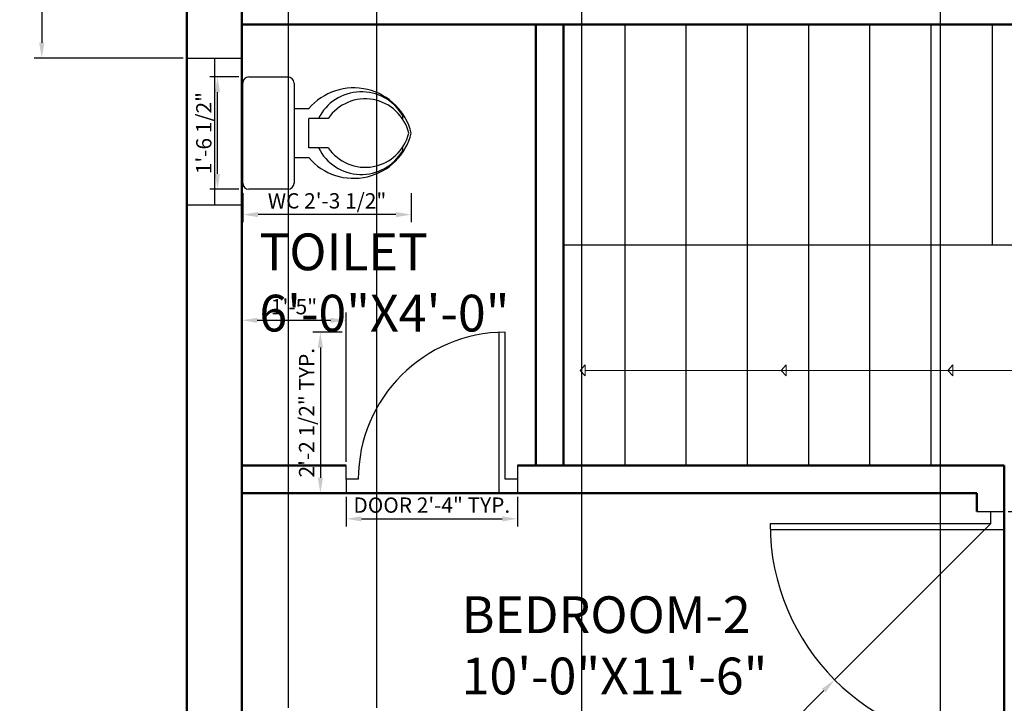
# Model space of a CAD drawing. Units: inches. Extents: x 3242 to 3618, y 1365 to 1814.
# Tile 2 of 6: x 3244 to 3405, y 1514 to 1626. Entities that reach past the tile are written whole.
import ezdxf

# ---------------------------------------------------------------- set-up
doc = ezdxf.new("R2010")
doc.units = ezdxf.units.IN
for name, color, linetype, lineweight in [('A-ANNO-DIMS', 2, 'Continuous', 18), ('A-ANNO-SYMB', 7, 'Continuous', 18), ('A-AREA-IDEN', 7, 'Continuous', 25), ('A-DOOR', 4, 'Continuous', 25), ('A-FLOR-FIXT', 8, 'Continuous', 25), ('A-FLOR-STRS', 7, 'Continuous', 25), ('A-GLAZ', 5, 'Continuous', 25), ('A-WALL', 7, 'Continuous', 50)]:
    doc.layers.add(name, color=color, linetype=linetype, lineweight=lineweight)
doc.styles.get("Standard").update_dxf_attribs({"font": 'arial.ttf'})
doc.dimstyles.new('ISO-25', dxfattribs={"dimtxt": 2.5, "dimasz": 2.5, "dimexe": 1.25, "dimexo": 0.625, "dimtad": 1, "dimdec": 0, "dimlunit": 3, "dimtxsty": 'Standard', "dimcen": 2.5, "dimadec": 0, "dimazin": 0, "dimtfac": 1, "dimtdec": 0, "dimtmove": 0, "dimatfit": 3, "dimfxl": 1, "dimarcsym": 0})

# ---------------------------------------------------------------- blocks, each defined once
blk = doc.blocks.new('A$C02F3725D')
for p, q in [((0.025, 0.69), (0.435, 0.69)), ((0, 0.505), (0, 0.665)), ((0.46, 0.665), (0.46, 0.505)), ((0.435, 0.48), (0.025, 0.48)), ((0.13, 0.48), (0.13, 0.42)), ((0.33, 0.42), (0.33, 0.48)), ((0.17, 0.34), (0.17, 0.42)), ((0.17, 0.42), (0.29, 0.42)), ((0.29, 0.34), (0.29, 0.42)), ((0.1578, 0.035), (0.1724, 0.035)), ((0.2876, 0.035), (0.3022, 0.035))]:
    blk.add_line(p, q)
for centre, radius, start, end in [((0.025, 0.665), 0.025, 90, 180), ((0.435, 0.665), 0.025, 0, 90), ((0.025, 0.505), 0.025, 180, 270), ((0.435, 0.505), 0.025, 270, 0), ((0.2874, 0.2356), 0.2425, 130.4885, 256.2965), ((0.1726, 0.2356), 0.2425, 283.7035, 49.5115), ((0.2568, 0.2042), 0.196, 116.2742, 239.6668), ((0.2032, 0.2042), 0.196, 300.3332, 63.7258), ((0.2732, 0.1883), 0.1834, 124.2157, 256.394), ((0.1868, 0.1883), 0.1834, 283.606, 55.7843)]:
    blk.add_arc(centre, radius, start, end)
blk = doc.blocks.new('DOOR-SWING-24IN')
for p, q in [((21.75, 28), (26.25, 28)), ((24, 28), (24, 26)), ((24, 26), (0, 26)), ((26.25, 25), (0, 25)), ((24, 2), (24, 0)), ((24, 0), (21.75, 0)), ((24, 0), (26.25, 0))]:
    blk.add_line(p, q)
blk.add_arc((24, 26), 24, 180, 270)
blk = doc.blocks.new('DOOR-SWING-36IN')
for p, q in [((33.75, 40), (38.25, 40)), ((36, 40), (36, 38)), ((36, 38), (0, 38)), ((38.25, 37), (0, 37)), ((36, 2), (36, 0)), ((36, 0), (33.75, 0)), ((36, 0), (38.25, 0))]:
    blk.add_line(p, q)
blk.add_arc((36, 38), 36, 180, 270)
blk = doc.blocks.new('WINDOW-24IN')
for p, q in [((0, 9), (24, 9)), ((0, 0), (0, 9)), ((24, 9), (24, 0)), ((0, 4.5), (24, 4.5)), ((24, 0), (0, 0))]:
    blk.add_line(p, q)
blk = doc.blocks.new('STAIR-DIR-ARROWHEAD')
for p, q in [((0.84, 1.76), (0, 0.88)), ((0.84, 0.88), (0.84, 1.76)), ((0.84, 0), (0, 0.88)), ((0.84, 0.88), (0.84, 0))]:
    blk.add_line(p, q)
blk = doc.blocks.new('*D17')
at = {"layer": 'A-ANNO-DIMS', "color": 0, "lineweight": -2, "transparency": 16777216}
for p, q in [((3405.61, 1545.66), (3412.23, 1545.66)), ((3410.98, 1508.16), (3410.98, 1543.16)), ((3405.61, 1505.66), (3412.23, 1505.66))]:
    blk.add_line(p, q, dxfattribs=at)
at = {"layer": 'A-ANNO-DIMS', "color": 0, "transparency": 16777216}
for points in [[(3410.56, 1543.16), (3411.4, 1543.16), (3410.98, 1545.66)], [(3410.56, 1508.16), (3411.4, 1508.16), (3410.98, 1505.66)]]:
    blk.add_solid(points, dxfattribs=at)
at = {"layer": 'Defpoints', "color": 0, "transparency": 16777216}
for p in [(3404.98, 1545.66), (3410.98, 1545.66), (3404.98, 1505.66)]:
    blk.add_point(p, dxfattribs=at)
at = {"layer": 'A-ANNO-DIMS', "color": 0, "transparency": 16777216, "insert": (3409.06, 1525.66), "char_height": 2.5, "attachment_point": 5, "rotation": 90}
blk.add_mtext('DOOR 3\'-4" TYP.', dxfattribs=at)
blk = doc.blocks.new('*D19')
at = {"layer": 'A-ANNO-DIMS', "color": 0, "lineweight": -2, "transparency": 16777216}
for p, q in [((3297.48, 1548.03), (3297.48, 1543.21)), ((3325.48, 1548.03), (3325.48, 1543.21)), ((3299.98, 1544.46), (3322.98, 1544.46))]:
    blk.add_line(p, q, dxfattribs=at)
at = {"layer": 'A-ANNO-DIMS', "color": 0, "transparency": 16777216}
for points in [[(3299.98, 1544.87), (3299.98, 1544.04), (3297.48, 1544.46)], [(3322.98, 1544.87), (3322.98, 1544.04), (3325.48, 1544.46)]]:
    blk.add_solid(points, dxfattribs=at)
at = {"layer": 'Defpoints', "color": 0, "transparency": 16777216}
for p in [(3297.48, 1548.66), (3325.48, 1548.66), (3325.48, 1544.46)]:
    blk.add_point(p, dxfattribs=at)
at = {"layer": 'A-ANNO-DIMS', "color": 0, "transparency": 16777216, "insert": (3311.48, 1546.37), "char_height": 2.5, "attachment_point": 5}
blk.add_mtext('DOOR 2\'-4" TYP.', dxfattribs=at)
blk = doc.blocks.new('*D20')
at = {"layer": 'A-ANNO-DIMS', "color": 0, "lineweight": -2, "transparency": 16777216}
for p, q in [((3296.86, 1574.91), (3292.03, 1574.91)), ((3293.28, 1572.41), (3293.28, 1551.16)), ((3296.86, 1548.66), (3292.03, 1548.66))]:
    blk.add_line(p, q, dxfattribs=at)
at = {"layer": 'A-ANNO-DIMS', "color": 0, "transparency": 16777216}
for points in [[(3292.86, 1572.41), (3293.7, 1572.41), (3293.28, 1574.91)], [(3292.86, 1551.16), (3293.7, 1551.16), (3293.28, 1548.66)]]:
    blk.add_solid(points, dxfattribs=at)
at = {"layer": 'Defpoints', "color": 0, "transparency": 16777216}
for p in [(3297.48, 1574.91), (3293.28, 1548.66), (3297.48, 1548.66)]:
    blk.add_point(p, dxfattribs=at)
at = {"layer": 'A-ANNO-DIMS', "color": 0, "transparency": 16777216, "insert": (3291.36, 1561.78), "char_height": 2.5, "attachment_point": 5, "rotation": 90}
blk.add_mtext('2\'-2 1/2" TYP.', dxfattribs=at)
blk = doc.blocks.new('*D23')
at = {"layer": 'A-ANNO-DIMS', "color": 0, "lineweight": -2, "transparency": 16777216}
for p, q in [((3280.61, 1597.61), (3280.61, 1592.86)), ((3308.12, 1597.61), (3308.12, 1592.86)), ((3305.62, 1594.11), (3283.11, 1594.11))]:
    blk.add_line(p, q, dxfattribs=at)
at = {"layer": 'A-ANNO-DIMS', "color": 0, "transparency": 16777216}
for points in [[(3283.11, 1594.53), (3283.11, 1593.69), (3280.61, 1594.11)], [(3305.62, 1594.53), (3305.62, 1593.69), (3308.12, 1594.11)]]:
    blk.add_solid(points, dxfattribs=at)
at = {"layer": 'Defpoints', "color": 0, "transparency": 16777216}
for p in [(3280.61, 1598.24), (3308.12, 1598.24), (3280.61, 1594.11)]:
    blk.add_point(p, dxfattribs=at)
at = {"layer": 'A-ANNO-DIMS', "color": 0, "transparency": 16777216, "insert": (3294.37, 1596.03), "char_height": 2.5, "attachment_point": 5}
blk.add_mtext('WC 2\'-3 1/2"', dxfattribs=at)
blk = doc.blocks.new('*D24')
at = {"layer": 'A-ANNO-DIMS', "color": 0, "lineweight": -2, "transparency": 16777216}
for p, q in [((3279.99, 1616.58), (3275.24, 1616.58)), ((3276.49, 1600.74), (3276.49, 1614.08)), ((3279.99, 1598.24), (3275.24, 1598.24))]:
    blk.add_line(p, q, dxfattribs=at)
at = {"layer": 'A-ANNO-DIMS', "color": 0, "transparency": 16777216}
for points in [[(3276.07, 1614.08), (3276.9, 1614.08), (3276.49, 1616.58)], [(3276.07, 1600.74), (3276.9, 1600.74), (3276.49, 1598.24)]]:
    blk.add_solid(points, dxfattribs=at)
at = {"layer": 'Defpoints', "color": 0, "transparency": 16777216}
for p in [(3276.49, 1616.58), (3280.61, 1616.58), (3280.61, 1598.24)]:
    blk.add_point(p, dxfattribs=at)
at = {"layer": 'A-ANNO-DIMS', "color": 0, "transparency": 16777216, "insert": (3274.57, 1607.41), "char_height": 2.5, "attachment_point": 5, "rotation": 90}
blk.add_mtext('1\'-6 1/2"', dxfattribs=at)
blk = doc.blocks.new('*D38')
at = {"layer": 'A-ANNO-DIMS', "color": 0, "lineweight": -2, "transparency": 16777216}
for p, q in [((3270.86, 1688.77), (3246.53, 1688.77)), ((3247.78, 1686.27), (3247.78, 1622.15)), ((3270.86, 1619.65), (3246.53, 1619.65))]:
    blk.add_line(p, q, dxfattribs=at)
at = {"layer": 'A-ANNO-DIMS', "color": 0, "transparency": 16777216}
for points in [[(3247.36, 1686.27), (3248.2, 1686.27), (3247.78, 1688.77)], [(3247.36, 1622.15), (3248.2, 1622.15), (3247.78, 1619.65)]]:
    blk.add_solid(points, dxfattribs=at)
at = {"layer": 'Defpoints', "color": 0, "transparency": 16777216}
for p in [(3271.48, 1688.77), (3247.78, 1619.65), (3271.48, 1619.65)]:
    blk.add_point(p, dxfattribs=at)
at = {"layer": 'A-ANNO-DIMS', "color": 0, "transparency": 16777216, "insert": (3245.88, 1654.21), "char_height": 2.5, "attachment_point": 5, "rotation": 90}
blk.add_mtext('5\'-9"', dxfattribs=at)
blk = doc.blocks.new('*D48')
at = {"layer": 'A-ANNO-DIMS', "color": 0, "lineweight": -2, "transparency": 16777216}
for p, q in [((3394.48, 1651.75), (3394.48, 1376.71)), ((3335.91, 1642.66), (3335.91, 1376.71)), ((3338.41, 1377.96), (3391.98, 1377.96))]:
    blk.add_line(p, q, dxfattribs=at)
at = {"layer": 'A-ANNO-DIMS', "color": 0, "transparency": 16777216}
for points in [[(3338.41, 1378.37), (3338.41, 1377.54), (3335.91, 1377.96)], [(3391.98, 1378.37), (3391.98, 1377.54), (3394.48, 1377.96)]]:
    blk.add_solid(points, dxfattribs=at)
at = {"layer": 'Defpoints', "color": 0, "transparency": 16777216}
for p in [(3394.48, 1652.37), (3335.91, 1643.28), (3394.48, 1377.96)]:
    blk.add_point(p, dxfattribs=at)
at = {"layer": 'A-ANNO-DIMS', "color": 0, "transparency": 16777216, "insert": (3365.2, 1379.87), "char_height": 2.5, "attachment_point": 5}
blk.add_mtext('4\'-10 1/2"', dxfattribs=at)
blk = doc.blocks.new('*D56')
at = {"layer": 'A-ANNO-DIMS', "color": 0, "lineweight": -2, "transparency": 16777216}
for p, q in [((3288.1, 1513.62), (3288.1, 1783.61)), ((3302.5, 1513.62), (3302.5, 1783.61)), ((3290.6, 1782.36), (3300, 1782.36))]:
    blk.add_line(p, q, dxfattribs=at)
at = {"layer": 'A-ANNO-DIMS', "color": 0, "transparency": 16777216}
for points in [[(3290.6, 1782.77), (3290.6, 1781.94), (3288.1, 1782.36)], [(3300, 1782.77), (3300, 1781.94), (3302.5, 1782.36)]]:
    blk.add_solid(points, dxfattribs=at)
at = {"layer": 'Defpoints', "color": 0, "transparency": 16777216}
for p in [(3302.5, 1782.36), (3288.1, 1513), (3302.5, 1513)]:
    blk.add_point(p, dxfattribs=at)
at = {"layer": 'A-ANNO-DIMS', "color": 0, "transparency": 16777216, "insert": (3295.3, 1784.27), "char_height": 2.5, "attachment_point": 5}
blk.add_mtext('1\'-2 1/2"', dxfattribs=at)
blk = doc.blocks.new('*D64')
at = {"layer": 'A-ANNO-DIMS', "color": 0, "lineweight": -2, "transparency": 16777216}
for p, q in [((3280.48, 1553.78), (3280.48, 1578.11)), ((3297.48, 1553.78), (3297.48, 1578.11)), ((3282.98, 1576.86), (3294.98, 1576.86))]:
    blk.add_line(p, q, dxfattribs=at)
at = {"layer": 'A-ANNO-DIMS', "color": 0, "transparency": 16777216}
for points in [[(3282.98, 1577.27), (3282.98, 1576.44), (3280.48, 1576.86)], [(3294.98, 1577.27), (3294.98, 1576.44), (3297.48, 1576.86)]]:
    blk.add_solid(points, dxfattribs=at)
at = {"layer": 'Defpoints', "color": 0, "transparency": 16777216}
for p in [(3297.48, 1576.86), (3280.48, 1553.16), (3297.48, 1553.16)]:
    blk.add_point(p, dxfattribs=at)
at = {"layer": 'A-ANNO-DIMS', "color": 0, "transparency": 16777216, "insert": (3288.98, 1578.76), "char_height": 2.5, "attachment_point": 5}
blk.add_mtext('1\'-5"', dxfattribs=at)
blk = doc.blocks.new('*D65')
at = {"layer": 'A-ANNO-DIMS', "color": 0, "lineweight": -2, "transparency": 16777216}
for p, q in [((3402.73, 1543.66), (3377.27, 1518.2)), ((3356.46, 1497.39), (3375.51, 1516.43))]:
    blk.add_line(p, q, dxfattribs=at)
at = {"layer": 'A-ANNO-DIMS', "color": 0, "transparency": 16777216}
blk.add_solid([(3375.21, 1516.73), (3375.8, 1516.14), (3377.27, 1518.2)], dxfattribs=at)
at = {"layer": 'Defpoints', "color": 0, "transparency": 16777216}
for p in [(3402.73, 1543.66), (3377.27, 1518.2)]:
    blk.add_point(p, dxfattribs=at)
at = {"layer": 'A-ANNO-DIMS', "color": 0, "transparency": 16777216, "insert": (3360.66, 1504.27), "char_height": 2.5, "attachment_point": 5, "rotation": 44.9992}
blk.add_mtext('3X R3\'-0"', dxfattribs=at)

msp = doc.modelspace()

# ---------------------------------------------------------------- linework, layer by layer
at = {"layer": 'A-ANNO-SYMB'}
msp.add_line((3407.4, 1568.69), (3336.54, 1568.69), dxfattribs=at)
at = {"layer": 'A-FLOR-STRS'}
for p, q in [((3342.98, 1625.16), (3342.98, 1553.16)), ((3352.98, 1625.16), (3352.98, 1553.16)), ((3362.98, 1625.16), (3362.98, 1553.16)), ((3372.98, 1625.16), (3372.98, 1553.16)), ((3382.98, 1625.16), (3382.98, 1553.16)), ((3392.98, 1625.16), (3392.98, 1553.16)), ((3402.98, 1625.16), (3402.98, 1589.16)), ((3332.98, 1589.16), (3442.98, 1589.16))]:
    msp.add_line(p, q, dxfattribs=at)
at = {"layer": 'A-WALL'}
for p, q in [((3271.48, 1758.66), (3271.48, 1401.66)), ((3280.48, 1749.66), (3280.48, 1410.66)), ((3280.48, 1625.16), (3463.48, 1625.16)), ((3328.48, 1625.16), (3328.48, 1553.16)), ((3332.98, 1625.16), (3332.98, 1553.16)), ((3280.48, 1553.16), (3297.48, 1553.16)), ((3325.48, 1553.16), (3404.98, 1553.16)), ((3404.98, 1553.16), (3404.98, 1410.66)), ((3280.48, 1548.66), (3400.48, 1548.66)), ((3400.48, 1548.66), (3400.48, 1545.66))]:
    msp.add_line(p, q, dxfattribs=at)

# ---------------------------------------------------------------- block references
at = {"layer": 'A-ANNO-SYMB'}
for p in [(3335.7, 1567.81), (3368.52, 1567.81), (3395.75, 1567.81)]:
    msp.add_blockref('STAIR-DIR-ARROWHEAD', p, dxfattribs=at)
at = {"layer": 'A-DOOR', "rotation": 270}
msp.add_blockref('DOOR-SWING-24IN', (3297.48, 1574.91), dxfattribs=at)
at = {"layer": 'A-DOOR'}
msp.add_blockref('DOOR-SWING-36IN', (3366.73, 1505.65), dxfattribs=at)
at = {"layer": 'A-FLOR-FIXT', "xscale": 39.87103032105172, "yscale": 39.87103032105172, "zscale": 39.87103032105172, "rotation": 90}
msp.add_blockref('A$C02F3725D', (3308.12, 1598.24), dxfattribs=at)
at = {"layer": 'A-GLAZ', "rotation": 270.0000000000009}
msp.add_blockref('WINDOW-24IN', (3271.48, 1619.65), dxfattribs=at)

# ---------------------------------------------------------------- texts
at = {"layer": 'A-AREA-IDEN', "char_height": 6, "attachment_point": 1}
for s, insert in [('TOILET\\P6\'-0"X4\'-0"', (3283.31, 1591.03)), ('BEDROOM-2\\P10\'-0"X11\'-6"', (3316.35, 1531.81))]:
    msp.add_mtext(s, dxfattribs=dict(at, insert=insert))

# ---------------------------------------------------------------- dimensions: what is measured, and where the dimension line sits
at = {"layer": 'A-ANNO-DIMS'}
for base, p1, p2, picture, middle in [((3302.5, 1782.36), (3288.1, 1513), (3302.5, 1513), '*D56', (3295.3, 1784.27)), ((3394.48, 1377.96), (3335.91, 1643.28), (3394.48, 1652.37), '*D48', (3365.2, 1379.87)), ((3297.48, 1576.86), (3280.48, 1553.16), (3297.48, 1553.16), '*D64', (3288.98, 1578.76))]:
    dim = msp.add_linear_dim(base=base, p1=p1, p2=p2, dimstyle='ISO-25', override={"dimdec": 1, "dimlfac": 1, "dimrnd": 0, "dimzin": 1, "dimdsep": 46, "dimlunit": 4, "dimfrac": 2}, dxfattribs=at)
    dim.commit()
    dim.dimension.update_dxf_attribs({"geometry": picture, "text_midpoint": middle})
for base, p1, p2, picture, middle in [((3247.78, 1619.65), (3271.48, 1688.77), (3271.48, 1619.65), '*D38', (3245.88, 1654.21)), ((3276.49, 1616.58), (3280.61, 1598.24), (3280.61, 1616.58), '*D24', (3274.57, 1607.41))]:
    dim = msp.add_linear_dim(base=base, p1=p1, p2=p2, angle=90, dimstyle='ISO-25', override={"dimdec": 1, "dimlfac": 1, "dimrnd": 0, "dimzin": 1, "dimdsep": 46, "dimlunit": 4, "dimfrac": 2}, dxfattribs=at)
    dim.commit()
    dim.dimension.update_dxf_attribs({"geometry": picture, "text_midpoint": middle})
for base, p1, p2, angle, text, picture, middle in [((3280.61, 1594.11), (3308.12, 1598.24), (3280.61, 1598.24), 180, 'WC <>', '*D23', (3294.37, 1596.03)), ((3293.28013858, 1548.65543785), (3297.48013858, 1574.90543785), (3297.48013858, 1548.65543785), 270, '<> TYP.', '*D20', (3291.36250556, 1561.78043785)), ((3410.98, 1545.66), (3404.98, 1505.66), (3404.98, 1545.66), 90, 'DOOR <> TYP.', '*D17', (3409.06, 1525.66))]:
    dim = msp.add_linear_dim(base=base, p1=p1, p2=p2, angle=angle, text=text, dimstyle='ISO-25', override={"dimdec": 1, "dimlfac": 1, "dimrnd": 0, "dimzin": 1, "dimdsep": 46, "dimlunit": 4, "dimfrac": 2}, dxfattribs=at)
    dim.commit()
    dim.dimension.update_dxf_attribs({"geometry": picture, "text_midpoint": middle})
dim = msp.add_linear_dim(base=(3325.48, 1544.46), p1=(3297.48, 1548.66), p2=(3325.48, 1548.66), text='DOOR <> TYP.', dimstyle='ISO-25', override={"dimdec": 1, "dimlfac": 1, "dimrnd": 0, "dimzin": 1, "dimdsep": 46, "dimlunit": 4, "dimfrac": 2}, dxfattribs=at)
dim.commit()
dim.dimension.update_dxf_attribs({"geometry": '*D19', "text_midpoint": (3311.48, 1546.37)})
dim = msp.add_radius_dim(center=(3402.73, 1543.66), mpoint=(3377.27, 1518.2), text='3X <>', dimstyle='ISO-25', override={"dimdec": 1, "dimlfac": 1, "dimrnd": 0, "dimzin": 1, "dimdsep": 46, "dimlunit": 4, "dimfrac": 2}, dxfattribs=at)
dim.commit()
dim.dimension.update_dxf_attribs({"geometry": '*D65', "text_midpoint": (3362, 1502.93), "dimtype": 164})

doc.saveas('drawing.dxf')
